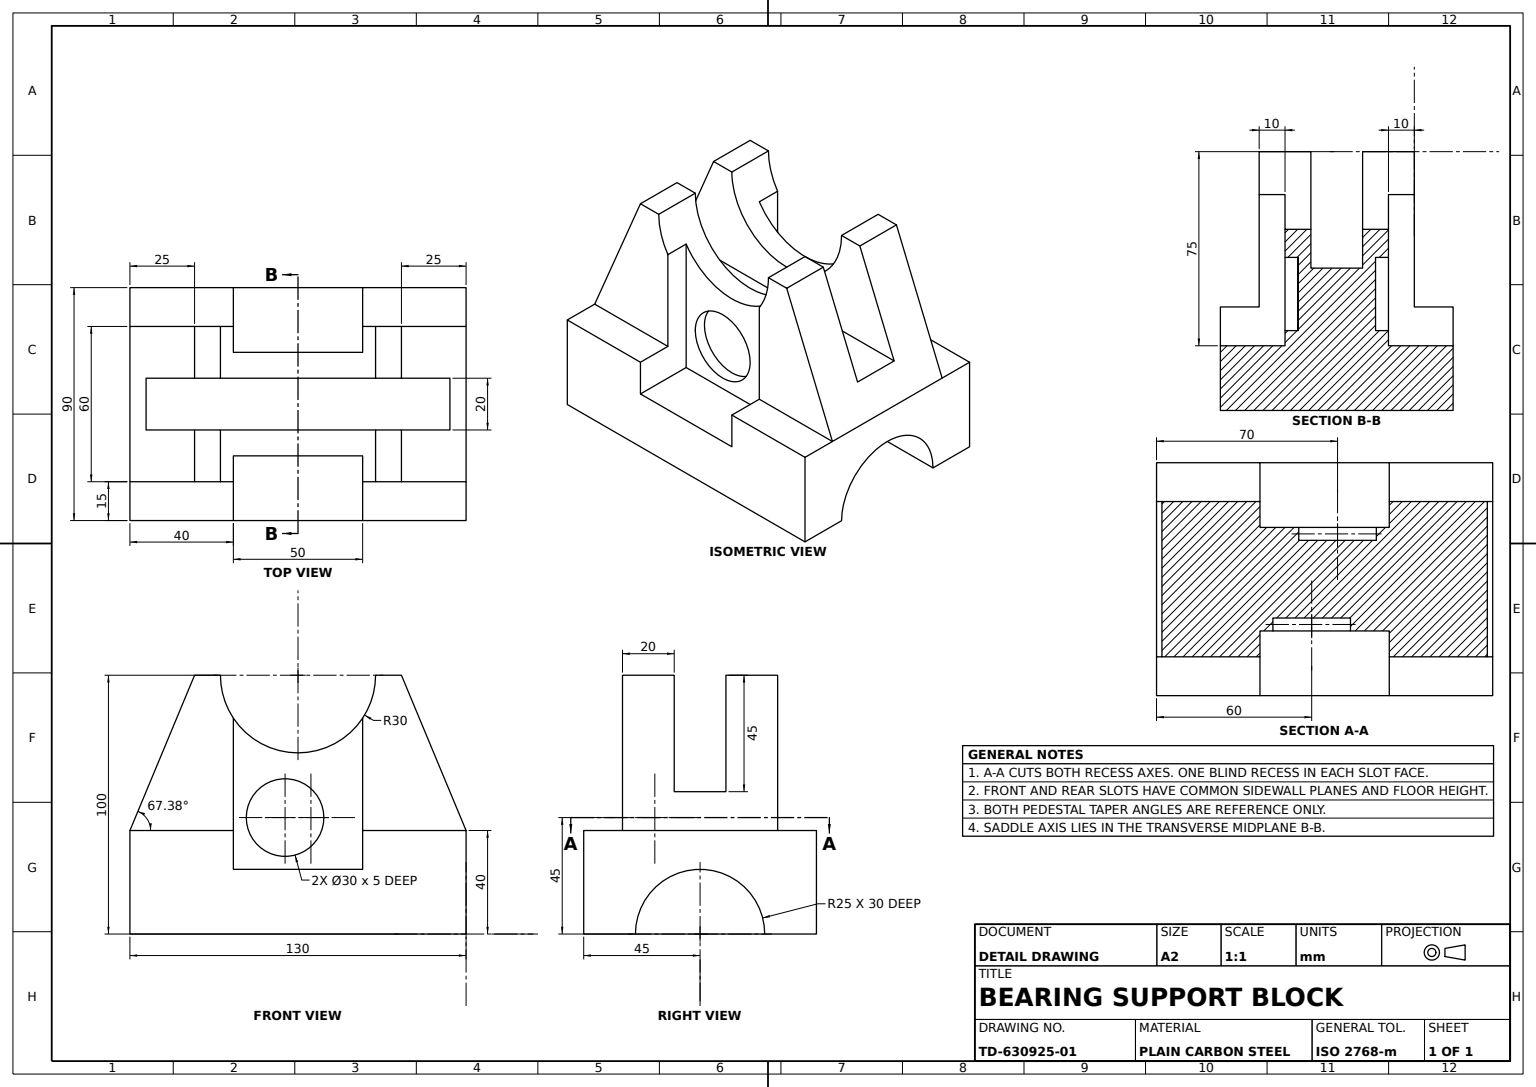
from build123d import *

# Parameters (mm, degrees)
BASE_BLOCK_DEPTH        = 45
BOTTOM_ARCH_CUT_DEPTH   = 30
BEARING_PEDESTAL_DEPTH  = 75
PEDESTAL_SIDE_CUT_DEPTH = 15
BEARING_SEAT_PROFILE_W  = 130
BEARING_SEAT_PROFILE_H  = 20
BEARING_SEAT_CUT_DEPTH  = 45
CROSS_HOLE_DEPTH        = 114.468057179
CROSS_HOLE_DEPTH_BACK   = 114.468057179
SLOT_A_CUT_DEPTH        = 10
SLOT_START              = -10
SLOT_B_CUT_DEPTH        = 10
STEP_RECESS_A_PROFILE_R = 15
STEP_RECESS_A_DEPTH     = 5
STEP_RECESS_B_PROFILE_R = 15
STEP_RECESS_B_DEPTH     = 5


with BuildPart() as part:
    # Base Block Profile → Base Block (new, symmetric)
    with BuildSketch(Plane.XY):
        Polygon((0, 0), (25, 0), (25, 15), (65, 15), (65, -25), (-65, -25), (-65, 15), (-25, 15), (-25, 0), align=None)
    extrude(amount=BASE_BLOCK_DEPTH, both=True)

    # Bottom Arch Profile R25 → Bottom Arch Cut (cut)
    with BuildSketch(Plane(origin=(65, 0, 0), x_dir=(0, 0, -1), z_dir=(1, 0, 0))):
        with BuildLine():
            Line((-25, -25), (25, -25))
            ThreePointArc((25, -25), (0, 0), (-25, -25))
        make_face()
    extrude(amount=-BOTTOM_ARCH_CUT_DEPTH, mode=Mode.SUBTRACT)

    # Pedestal Profile → Bearing Pedestal (add)
    with BuildSketch(Plane.XY.offset(45)):
        Polygon((-65, 15), (-40, 75), (40, 75), (65, 15), (25, 15), (25, 0), (-25, 0), (-25, 15), align=None)
    extrude(amount=-BEARING_PEDESTAL_DEPTH)

    # Pedestal Side Cut Profile → Pedestal Side Cut (cut)
    with BuildSketch(Plane.XY.offset(45)):
        Polygon((-65, 15), (-25, 15), (-25, 0), (25, 0), (25, 15), (65, 15), (40, 75), (-40, 75), align=None)
    extrude(amount=-PEDESTAL_SIDE_CUT_DEPTH, mode=Mode.SUBTRACT)

    # Bearing Seat Profile → Bearing Seat Cut (cut)
    with BuildSketch(Plane(origin=(0, 75, 0), x_dir=(1, 0, 0), z_dir=(0, 1, 0))):
        Rectangle(BEARING_SEAT_PROFILE_W, BEARING_SEAT_PROFILE_H)
    extrude(amount=-BEARING_SEAT_CUT_DEPTH, mode=Mode.SUBTRACT)

    # Cross Hole Profile → Cross Hole (cut, two sides: drawn at the far end of the back side and taken through both)
    with BuildSketch(Plane(origin=(0, 0, 10), x_dir=(-1, 0, 0), z_dir=(0, 0, -1)).offset(-CROSS_HOLE_DEPTH_BACK)):
        with BuildLine():
            Line((-30, 75), (30, 75))
            ThreePointArc((30, 75), (0, 45), (-30, 75))
        make_face()
    extrude(amount=CROSS_HOLE_DEPTH + CROSS_HOLE_DEPTH_BACK, mode=Mode.SUBTRACT)

    # Slot A Profile → Slot A Cut (cut)
    with BuildSketch(Plane.XY.offset(30)):
        with BuildLine():
            Line((-25, 0), (-25, 58.416876048))
            ThreePointArc((-25, 58.416876048), (0, 45), (25, 58.416876048))
            Line((25, 58.416876048), (25, 0))
            Line((25, 0), (-25, 0))
        make_face()
    extrude(amount=-SLOT_A_CUT_DEPTH, mode=Mode.SUBTRACT)

    # Slot B Profile → Slot B Cut (cut)
    with BuildSketch(Plane(origin=(0, 0, -30), x_dir=(-1, 0, 0), z_dir=(0, 0, -1)).offset(SLOT_START)):
        with BuildLine():
            Line((-25, 0), (25, 0))
            Line((25, 0), (25, 58.416876048))
            ThreePointArc((25, 58.416876048), (0, 45), (-25, 58.416876048))
            Line((-25, 58.416876048), (-25, 0))
        make_face()
    extrude(amount=SLOT_B_CUT_DEPTH, mode=Mode.SUBTRACT)

    # Step Recess A Profile → Step Recess A (cut)
    with BuildSketch(Plane(origin=(0, 0, -20), x_dir=(-1, 0, 0), z_dir=(0, 0, -1))):
        with Locations((-5, 20)):
            Circle(STEP_RECESS_A_PROFILE_R)
    extrude(amount=-STEP_RECESS_A_DEPTH, mode=Mode.SUBTRACT)

    # Step Recess B Profile → Step Recess B (cut)
    with BuildSketch(Plane.XY.offset(20)):
        with Locations((-5, 20)):
            Circle(STEP_RECESS_B_PROFILE_R)
    extrude(amount=-STEP_RECESS_B_DEPTH, mode=Mode.SUBTRACT)


solid = part.part
